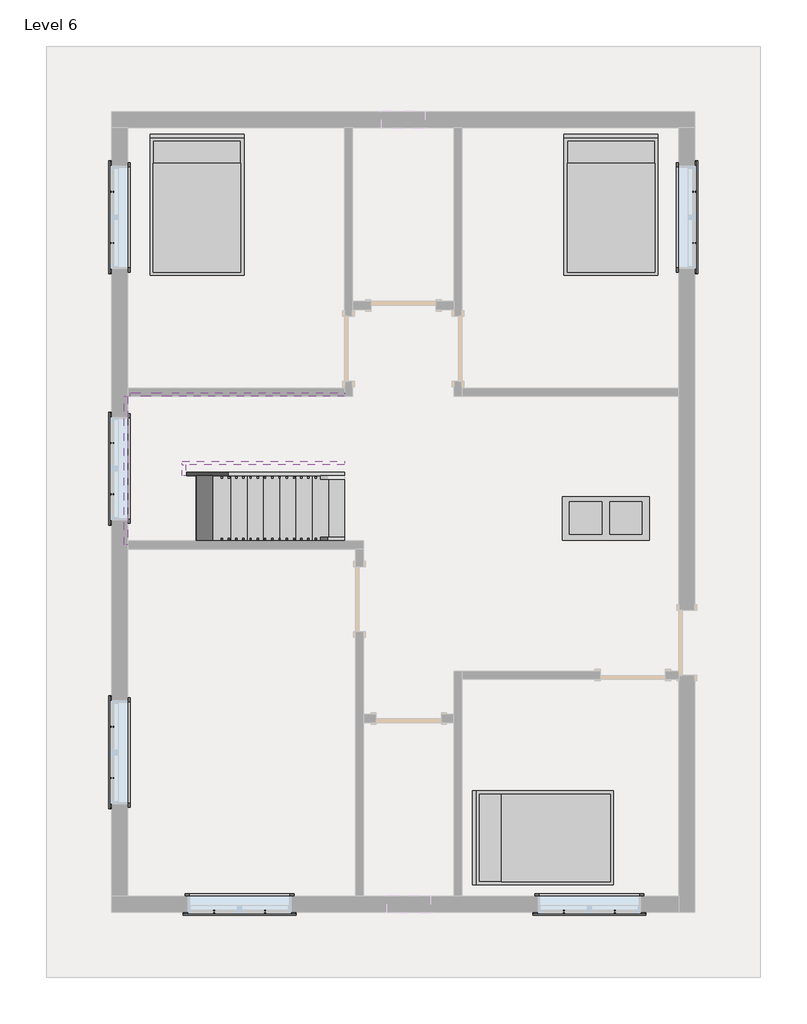
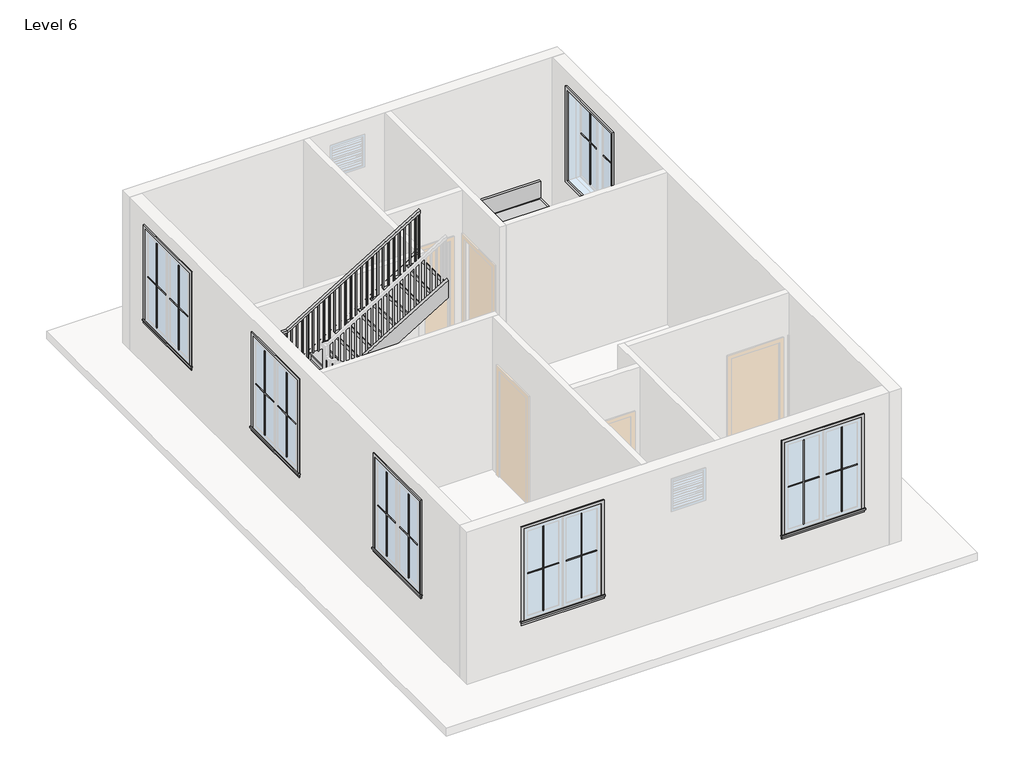
# One storey, part 2 of 2: 25 proxies, 6 members, 3 furniture elements, 1 railing, 1 stair flight.
"""IFC4 building model written with IfcOpenShell, lengths in millimetres."""

from ifc_helpers import new_model, si_unit, frame, origin, place, context, project, spatial, polyline, outline, extrude, faceted_brep, transform, mapped, element, save
from components import muntin_pattern_2x2_muntin_pattern_2x2_bff912c5, muntin_pattern_2x2_muntin_pattern_2x2_c2194282, trim_window_exterior_flat_with_sill_e04b3088, trim_window_interior_flat_picture_frame_2a7685fe, coffee_table_with_brass_mullions_11320_coffee_table_with_5962bef7, bed_17739_bed_17739_15c61121, stair_flight_418e8841

model = new_model("IFC4")

# Units and contexts
model_context = context("Model", 3, world=origin())
ifc_project = project(units=[si_unit("LENGTHUNIT", "METRE", prefix="MILLI")], contexts=[model_context])

# Site, building, storey
site = spatial("IfcSite", under=ifc_project)
building = spatial("IfcBuilding", under=site)
storey = spatial("IfcBuildingStorey", under=building, Name="Level 6", Elevation=12801.6)

# Proxies
placement = place(None, origin())
muntin_pattern_2x2_muntin_pattern_2x2_shape = muntin_pattern_2x2_muntin_pattern_2x2_bff912c5(model_context)
element("IfcBuildingElementProxy", 1, Name="Muntin Pattern_2x2 : Muntin Pattern_2x2", ObjectType="Muntin Pattern_2x2 : Muntin Pattern_2x2", at=placement, inside=storey, context=model_context, shape_type="MappedRepresentation", body=[
    mapped(muntin_pattern_2x2_muntin_pattern_2x2_shape, transform((-3196.8535855, -5792.3946383, 13785.85), x_axis=(-1.0, 0.0, 0.0), y_axis=(0.0, -1.0, 0.0), z_axis=(0.0, 0.0, 1.0))),
])
element("IfcBuildingElementProxy", 2, Name="Muntin Pattern_2x2 : Muntin Pattern_2x2", ObjectType="Muntin Pattern_2x2 : Muntin Pattern_2x2", at=placement, inside=storey, context=model_context, shape_type="MappedRepresentation", body=[
    mapped(muntin_pattern_2x2_muntin_pattern_2x2_shape, transform((-5347.9160855, -3914.3821383, 13785.85), x_axis=(0.0, 1.0, 0.0), y_axis=(-1.0, 0.0, 0.0), z_axis=(0.0, 0.0, 1.0))),
])
element("IfcBuildingElementProxy", 3, Name="Muntin Pattern_2x2 : Muntin Pattern_2x2", ObjectType="Muntin Pattern_2x2 : Muntin Pattern_2x2", at=placement, inside=storey, context=model_context, shape_type="MappedRepresentation", body=[
    mapped(muntin_pattern_2x2_muntin_pattern_2x2_shape, transform((1721.2214145, -5792.3946383, 13785.85), x_axis=(-1.0, 0.0, 0.0), y_axis=(0.0, -1.0, 0.0), z_axis=(0.0, 0.0, 1.0))),
])
element("IfcBuildingElementProxy", 4, Name="Muntin Pattern_2x2 : Muntin Pattern_2x2", ObjectType="Muntin Pattern_2x2 : Muntin Pattern_2x2", at=placement, inside=storey, context=model_context, shape_type="MappedRepresentation", body=[
    mapped(muntin_pattern_2x2_muntin_pattern_2x2_shape, transform((2837.2339145, 4324.7428617, 13785.85), x_axis=(0.0, -1.0, 0.0), y_axis=(1.0, 0.0, 0.0), z_axis=(0.0, 0.0, 1.0))),
])
element("IfcBuildingElementProxy", 5, Name="Muntin Pattern_2x2 : Muntin Pattern_2x2", ObjectType="Muntin Pattern_2x2 : Muntin Pattern_2x2", at=placement, inside=storey, context=model_context, shape_type="MappedRepresentation", body=[
    mapped(muntin_pattern_2x2_muntin_pattern_2x2_shape, transform((-5347.9160855, 3604.0178617, 13785.85), x_axis=(0.0, 1.0, 0.0), y_axis=(-1.0, 0.0, 0.0), z_axis=(0.0, 0.0, 1.0))),
])
element("IfcBuildingElementProxy", 6, Name="Muntin Pattern_2x2 : Muntin Pattern_2x2", ObjectType="Muntin Pattern_2x2 : Muntin Pattern_2x2", at=placement, inside=storey, context=model_context, shape_type="MappedRepresentation", body=[
    mapped(muntin_pattern_2x2_muntin_pattern_2x2_shape, transform((-5347.9160855, 73.4178617, 13785.85), x_axis=(0.0, 1.0, 0.0), y_axis=(-1.0, 0.0, 0.0), z_axis=(0.0, 0.0, 1.0))),
])
muntin_pattern_2x2_muntin_pattern_2x2_2_shape = muntin_pattern_2x2_muntin_pattern_2x2_c2194282(model_context)
element("IfcBuildingElementProxy", 7, Name="Muntin Pattern_2x2 : Muntin Pattern_2x2", ObjectType="Muntin Pattern_2x2 : Muntin Pattern_2x2", at=placement, inside=storey, context=model_context, shape_type="MappedRepresentation", body=[
    mapped(muntin_pattern_2x2_muntin_pattern_2x2_2_shape, transform((-3917.5785855, -5792.3946383, 13785.85), x_axis=(1.0, 0.0, 0.0), y_axis=(0.0, 1.0, 0.0), z_axis=(0.0, 0.0, 1.0))),
])
element("IfcBuildingElementProxy", 8, Name="Muntin Pattern_2x2 : Muntin Pattern_2x2", ObjectType="Muntin Pattern_2x2 : Muntin Pattern_2x2", at=placement, inside=storey, context=model_context, shape_type="MappedRepresentation", body=[
    mapped(muntin_pattern_2x2_muntin_pattern_2x2_2_shape, transform((-5347.9160855, -3193.6571383, 13785.85), x_axis=(0.0, -1.0, 0.0), y_axis=(1.0, 0.0, 0.0), z_axis=(0.0, 0.0, 1.0))),
])
element("IfcBuildingElementProxy", 9, Name="Muntin Pattern_2x2 : Muntin Pattern_2x2", ObjectType="Muntin Pattern_2x2 : Muntin Pattern_2x2", at=placement, inside=storey, context=model_context, shape_type="MappedRepresentation", body=[
    mapped(muntin_pattern_2x2_muntin_pattern_2x2_2_shape, transform((1000.4964145, -5792.3946383, 13785.85), x_axis=(1.0, 0.0, 0.0), y_axis=(0.0, 1.0, 0.0), z_axis=(0.0, 0.0, 1.0))),
])
element("IfcBuildingElementProxy", 10, Name="Muntin Pattern_2x2 : Muntin Pattern_2x2", ObjectType="Muntin Pattern_2x2 : Muntin Pattern_2x2", at=placement, inside=storey, context=model_context, shape_type="MappedRepresentation", body=[
    mapped(muntin_pattern_2x2_muntin_pattern_2x2_2_shape, transform((2837.2339145, 3604.0178617, 13785.85), x_axis=(0.0, 1.0, 0.0), y_axis=(-1.0, 0.0, 0.0), z_axis=(0.0, 0.0, 1.0))),
])
element("IfcBuildingElementProxy", 11, Name="Muntin Pattern_2x2 : Muntin Pattern_2x2", ObjectType="Muntin Pattern_2x2 : Muntin Pattern_2x2", at=placement, inside=storey, context=model_context, shape_type="MappedRepresentation", body=[
    mapped(muntin_pattern_2x2_muntin_pattern_2x2_2_shape, transform((-5347.9160855, 4324.7428617, 13785.85), x_axis=(0.0, -1.0, 0.0), y_axis=(1.0, 0.0, 0.0), z_axis=(0.0, 0.0, 1.0))),
])
element("IfcBuildingElementProxy", 12, Name="Muntin Pattern_2x2 : Muntin Pattern_2x2", ObjectType="Muntin Pattern_2x2 : Muntin Pattern_2x2", at=placement, inside=storey, context=model_context, shape_type="MappedRepresentation", body=[
    mapped(muntin_pattern_2x2_muntin_pattern_2x2_2_shape, transform((-5347.9160855, 794.1428617, 13785.85), x_axis=(0.0, -1.0, 0.0), y_axis=(1.0, 0.0, 0.0), z_axis=(0.0, 0.0, 1.0))),
])
trim_window_exterior_flat_with_sill_shape = trim_window_exterior_flat_with_sill_e04b3088(model_context)
element("IfcBuildingElementProxy", 13, Name="Trim-Window-Exterior-Flat : with Sill", ObjectType="Trim-Window-Exterior-Flat : with Sill", at=placement, inside=storey, context=model_context, shape_type="MappedRepresentation", body=[
    mapped(trim_window_exterior_flat_with_sill_shape, transform((-3557.2160855, -5801.9196383, 15544.8), x_axis=(1.0, 0.0, 0.0), y_axis=(0.0, 0.0, 1.0), z_axis=(0.0, -1.0, 0.0))),
])
element("IfcBuildingElementProxy", 14, Name="Trim-Window-Exterior-Flat : with Sill", ObjectType="Trim-Window-Exterior-Flat : with Sill", at=placement, inside=storey, context=model_context, shape_type="MappedRepresentation", body=[
    mapped(trim_window_exterior_flat_with_sill_shape, transform((-5357.4410855, -3554.0196383, 15544.8), x_axis=(0.0, -1.0, 0.0), y_axis=(0.0, 0.0, 1.0), z_axis=(-1.0, 0.0, 0.0))),
])
element("IfcBuildingElementProxy", 15, Name="Trim-Window-Exterior-Flat : with Sill", ObjectType="Trim-Window-Exterior-Flat : with Sill", at=placement, inside=storey, context=model_context, shape_type="MappedRepresentation", body=[
    mapped(trim_window_exterior_flat_with_sill_shape, transform((1360.8589145, -5801.9196383, 15544.8), x_axis=(1.0, 0.0, 0.0), y_axis=(0.0, 0.0, 1.0), z_axis=(0.0, -1.0, 0.0))),
])
element("IfcBuildingElementProxy", 16, Name="Trim-Window-Exterior-Flat : with Sill", ObjectType="Trim-Window-Exterior-Flat : with Sill", at=placement, inside=storey, context=model_context, shape_type="MappedRepresentation", body=[
    mapped(trim_window_exterior_flat_with_sill_shape, transform((2846.7589145, 3964.3803617, 15544.8), x_axis=(0.0, 1.0, 0.0), y_axis=(0.0, 0.0, 1.0), z_axis=(1.0, 0.0, 0.0))),
])
element("IfcBuildingElementProxy", 17, Name="Trim-Window-Exterior-Flat : with Sill", ObjectType="Trim-Window-Exterior-Flat : with Sill", at=placement, inside=storey, context=model_context, shape_type="MappedRepresentation", body=[
    mapped(trim_window_exterior_flat_with_sill_shape, transform((-5357.4410855, 3964.3803617, 15544.8), x_axis=(0.0, -1.0, 0.0), y_axis=(0.0, 0.0, 1.0), z_axis=(-1.0, 0.0, 0.0))),
])
element("IfcBuildingElementProxy", 18, Name="Trim-Window-Exterior-Flat : with Sill", ObjectType="Trim-Window-Exterior-Flat : with Sill", at=placement, inside=storey, context=model_context, shape_type="MappedRepresentation", body=[
    mapped(trim_window_exterior_flat_with_sill_shape, transform((-5357.4410855, 433.7803617, 15544.8), x_axis=(0.0, -1.0, 0.0), y_axis=(0.0, 0.0, 1.0), z_axis=(-1.0, 0.0, 0.0))),
])
trim_window_interior_flat_picture_frame_shape = trim_window_interior_flat_picture_frame_2a7685fe(model_context)
element("IfcBuildingElementProxy", 19, Name="Trim-Window-Interior-Flat : Picture Frame", ObjectType="Trim-Window-Interior-Flat : Picture Frame", at=placement, inside=storey, context=model_context, shape_type="MappedRepresentation", body=[
    mapped(trim_window_interior_flat_picture_frame_shape, transform((-3557.2160855, -5573.3196383, 15544.8), x_axis=(-1.0, 0.0, 0.0), y_axis=(0.0, 0.0, 1.0), z_axis=(0.0, 1.0, 0.0))),
])
element("IfcBuildingElementProxy", 20, Name="Trim-Window-Interior-Flat : Picture Frame", ObjectType="Trim-Window-Interior-Flat : Picture Frame", at=placement, inside=storey, context=model_context, shape_type="MappedRepresentation", body=[
    mapped(trim_window_interior_flat_picture_frame_shape, transform((-5128.8410855, -3554.0196383, 15544.8), x_axis=(0.0, 1.0, 0.0), y_axis=(0.0, 0.0, 1.0), z_axis=(1.0, 0.0, 0.0))),
])
element("IfcBuildingElementProxy", 21, Name="Trim-Window-Interior-Flat : Picture Frame", ObjectType="Trim-Window-Interior-Flat : Picture Frame", at=placement, inside=storey, context=model_context, shape_type="MappedRepresentation", body=[
    mapped(trim_window_interior_flat_picture_frame_shape, transform((1360.8589145, -5573.3196383, 15544.8), x_axis=(-1.0, 0.0, 0.0), y_axis=(0.0, 0.0, 1.0), z_axis=(0.0, 1.0, 0.0))),
])
element("IfcBuildingElementProxy", 22, Name="Trim-Window-Interior-Flat : Picture Frame", ObjectType="Trim-Window-Interior-Flat : Picture Frame", at=placement, inside=storey, context=model_context, shape_type="MappedRepresentation", body=[
    mapped(trim_window_interior_flat_picture_frame_shape, transform((2618.1589145, 3964.3803617, 15544.8), x_axis=(0.0, -1.0, 0.0), y_axis=(0.0, 0.0, 1.0), z_axis=(-1.0, 0.0, 0.0))),
])
element("IfcBuildingElementProxy", 23, Name="Trim-Window-Interior-Flat : Picture Frame", ObjectType="Trim-Window-Interior-Flat : Picture Frame", at=placement, inside=storey, context=model_context, shape_type="MappedRepresentation", body=[
    mapped(trim_window_interior_flat_picture_frame_shape, transform((-5128.8410855, 3964.3803617, 15544.8), x_axis=(0.0, 1.0, 0.0), y_axis=(0.0, 0.0, 1.0), z_axis=(1.0, 0.0, 0.0))),
])
element("IfcBuildingElementProxy", 24, Name="Trim-Window-Interior-Flat : Picture Frame", ObjectType="Trim-Window-Interior-Flat : Picture Frame", at=placement, inside=storey, context=model_context, shape_type="MappedRepresentation", body=[
    mapped(trim_window_interior_flat_picture_frame_shape, transform((-5128.8410855, 433.7803617, 15544.8), x_axis=(0.0, 1.0, 0.0), y_axis=(0.0, 0.0, 1.0), z_axis=(1.0, 0.0, 0.0))),
])
coffee_table_with_brass_mullions_11320_coffee_table_with_shape = coffee_table_with_brass_mullions_11320_coffee_table_with_5962bef7(model_context)
element("IfcBuildingElementProxy", 25, Name="coffee_table_with_brass_mullions_11320 : coffee_table_with_brass_mullions_11320", ObjectType="coffee_table_with_brass_mullions_11320 : coffee_table_with_brass_mullions_11320", at=placement, inside=storey, context=model_context, shape_type="MappedRepresentation", body=[
    mapped(coffee_table_with_brass_mullions_11320_coffee_table_with_shape, transform((2229.2258874, -696.5196383, 12801.6), x_axis=(1.0, 0.0, 0.0), y_axis=(0.0, 1.0, 0.0), z_axis=(0.0, 0.0, 1.0))),
])

# Furniture
bed_17739_bed_17739_shape = bed_17739_bed_17739_15c61121(model_context)
element("IfcFurniture", 26, ObjectType="Bed_17739 : Bed_17739", at=placement, inside=storey, context=model_context, shape_type="MappedRepresentation", body=[
    mapped(bed_17739_bed_17739_shape, transform((1665.6589145, 4116.7803617, 12801.6), x_axis=(1.0, 0.0, 0.0), y_axis=(0.0, 1.0, 0.0), z_axis=(0.0, 0.0, 1.0))),
])
element("IfcFurniture", 27, ObjectType="Bed_17739 : Bed_17739", at=placement, inside=storey, context=model_context, shape_type="MappedRepresentation", body=[
    mapped(bed_17739_bed_17739_shape, transform((-4157.2910855, 4116.7803617, 12801.6), x_axis=(1.0, 0.0, 0.0), y_axis=(0.0, 1.0, 0.0), z_axis=(0.0, 0.0, 1.0))),
])
element("IfcFurniture", 28, ObjectType="Bed_17739 : Bed_17739", at=placement, inside=storey, context=model_context, shape_type="MappedRepresentation", body=[
    mapped(bed_17739_bed_17739_shape, transform((732.2089145, -4754.5725945, 12801.6), x_axis=(0.0, 1.0, 0.0), y_axis=(-1.0, 0.0, 0.0), z_axis=(0.0, 0.0, 1.0))),
])

# Members
element("IfcMember", 29, ObjectType="Stringer - 2\" Width", at=placement, inside=storey, context=model_context, shape_type="SweptSolid", body=[
    extrude(outline(polyline([(12801.6, -2080.8410855), (13013.714512, -2080.8410855), (14401.8, -4371.1821407), (14401.8, -4959.2565972), (12801.6, -2318.9265972), (12801.6, -2080.8410855)])), frame((0.0, -633.0196383, 0.0), z_axis=(0.0, 1.0, 0.0), x_axis=(0.0, 0.0, 1.0)), (0.0, 0.0, 1.0), 50.8),
])
element("IfcMember", 30, ObjectType="Stringer - 2\" Width", at=placement, inside=storey, context=model_context, shape_type="SweptSolid", body=[
    extrude(outline(polyline([(-5128.8410855, -633.0196383), (-5179.6410855, -633.0196383), (-5179.6410855, 1449.7803617), (-5128.8410855, 1449.7803617), (-5128.8410855, -633.0196383)])), frame((0.0, 0.0, 14097.0), z_axis=(0.0, 0.0, 1.0), x_axis=(1.0, 0.0, 0.0)), (0.0, 0.0, 1.0), 304.8),
])
element("IfcMember", 31, ObjectType="Stringer - 2\" Width", at=placement, inside=storey, context=model_context, shape_type="SweptSolid", body=[
    extrude(outline(polyline([(14097.0, -4505.9455737), (15566.7602959, -2080.8410855), (15923.1690574, -2080.8410855), (14097.0, -5094.0200302), (14097.0, -4505.9455737)])), frame((0.0, 1449.7803617, 0.0), z_axis=(0.0, 1.0, 0.0), x_axis=(0.0, 0.0, 1.0)), (0.0, 0.0, 1.0), 50.8),
])
element("IfcMember", 32, ObjectType="Stringer - 2\" Width", at=placement, inside=storey, context=model_context, shape_type="SweptSolid", body=[
    extrude(outline(polyline([(12801.6, -2080.8410855), (13013.714512, -2080.8410855), (14368.3811786, -4316.0410855), (14011.9724171, -4316.0410855), (12801.6, -2318.9265972), (12801.6, -2080.8410855)])), frame((0.0, 332.1803617, 0.0), z_axis=(0.0, 1.0, 0.0), x_axis=(0.0, 0.0, 1.0)), (0.0, 0.0, 1.0), 50.8),
])
element("IfcMember", 33, ObjectType="Stringer - 2\" Width", at=placement, inside=storey, context=model_context, shape_type="SweptSolid", body=[
    extrude(outline(polyline([(-4316.0410855, 332.1803617), (-4366.8410855, 332.1803617), (-4366.8410855, 484.5803617), (-4316.0410855, 484.5803617), (-4316.0410855, 332.1803617)])), frame((0.0, 0.0, 14097.0), z_axis=(0.0, 0.0, 1.0), x_axis=(1.0, 0.0, 0.0)), (0.0, 0.0, 1.0), 304.8),
])
element("IfcMember", 34, ObjectType="Stringer - 2\" Width", at=placement, inside=storey, context=model_context, shape_type="SweptSolid", body=[
    extrude(outline(polyline([(14537.714512, -4366.8410855), (14181.3057504, -4366.8410855), (15566.7602959, -2080.8410855), (15923.1690574, -2080.8410855), (14537.714512, -4366.8410855)])), frame((0.0, 484.5803617, 0.0), z_axis=(0.0, 1.0, 0.0), x_axis=(0.0, 0.0, 1.0)), (0.0, 0.0, 1.0), 50.8),
])

# Railing
element("IfcRailing", 35, ObjectType="Handrail - Rectangular", at=placement, inside=storey, context=model_context, shape_type="SolidModel", body=[
    faceted_brep([(-2080.8410855, -582.2196383, 13854.5454545), (-2080.8410855, -582.2196383, 13795.1439943), (-2080.8410855, -531.4196383, 13795.1439943), (-2080.8410855, -531.4196383, 13854.5454545), (-4366.8410855, -582.2196383, 15240.0), (-4381.0334949, -582.2196383, 15189.2), (-4381.0334949, -531.4196383, 15189.2), (-4366.8410855, -531.4196383, 15240.0), (-5128.8410855, -582.2196383, 15240.0), (-5128.8410855, -582.2196383, 15189.2), (-5078.0410855, -531.4196383, 15189.2), (-5078.0410855, -531.4196383, 15240.0), (-5128.8410855, 1449.7803617, 15240.0), (-5128.8410855, 1449.7803617, 15189.2), (-5078.0410855, 1398.9803617, 15189.2), (-5078.0410855, 1398.9803617, 15240.0), (-4595.4410855, 1449.7803617, 15240.0), (-4581.2486761, 1449.7803617, 15189.2), (-4581.2486761, 1398.9803617, 15189.2), (-4595.4410855, 1398.9803617, 15240.0), (-2080.8410855, 1449.7803617, 16764.0), (-2080.8410855, 1398.9803617, 16764.0), (-2080.8410855, 1398.9803617, 16704.5985397), (-2080.8410855, 1449.7803617, 16704.5985397)], [[[0, 1, 2, 3]], [[1, 0, 4, 5]], [[2, 1, 5, 6]], [[3, 2, 6, 7]], [[0, 3, 7, 4]], [[5, 4, 8, 9]], [[6, 5, 9, 10]], [[7, 6, 10, 11]], [[4, 7, 11, 8]], [[9, 8, 12, 13]], [[10, 9, 13, 14]], [[11, 10, 14, 15]], [[8, 11, 15, 12]], [[13, 12, 16, 17]], [[14, 13, 17, 18]], [[15, 14, 18, 19]], [[12, 15, 19, 16]], [[20, 21, 22, 23]], [[17, 16, 20, 23]], [[18, 17, 23, 22]], [[19, 18, 22, 21]], [[16, 19, 21, 20]]]),
    extrude(outline(polyline([(16652.6439943, -2166.5660855), (15711.0545455, -2166.5660855), (15711.0545455, -2147.5160855), (16664.1894488, -2147.5160855), (16652.6439943, -2166.5660855)])), frame((0.0, 1414.8553617, 0.0), z_axis=(0.0, 1.0, 0.0), x_axis=(0.0, 0.0, 1.0)), (0.0, 0.0, 1.0), 19.05),
    extrude(outline(polyline([(16591.0682367, -2268.1660855), (15711.0545455, -2268.1660855), (15711.0545455, -2249.1160855), (16602.6136913, -2249.1160855), (16591.0682367, -2268.1660855)])), frame((0.0, 1414.8553617, 0.0), z_axis=(0.0, 1.0, 0.0), x_axis=(0.0, 0.0, 1.0)), (0.0, 0.0, 1.0), 19.05),
    extrude(outline(polyline([(16529.4924791, -2369.7660855), (15572.5090909, -2369.7660855), (15572.5090909, -2350.7160855), (16541.0379337, -2350.7160855), (16529.4924791, -2369.7660855)])), frame((0.0, 1414.8553617, 0.0), z_axis=(0.0, 1.0, 0.0), x_axis=(0.0, 0.0, 1.0)), (0.0, 0.0, 1.0), 19.05),
    extrude(outline(polyline([(16467.9167216, -2471.3660855), (15572.5090909, -2471.3660855), (15572.5090909, -2452.3160855), (16479.4621761, -2452.3160855), (16467.9167216, -2471.3660855)])), frame((0.0, 1414.8553617, 0.0), z_axis=(0.0, 1.0, 0.0), x_axis=(0.0, 0.0, 1.0)), (0.0, 0.0, 1.0), 19.05),
    extrude(outline(polyline([(16406.340964, -2572.9660855), (15433.9636364, -2572.9660855), (15433.9636364, -2553.9160855), (16417.8864185, -2553.9160855), (16406.340964, -2572.9660855)])), frame((0.0, 1414.8553617, 0.0), z_axis=(0.0, 1.0, 0.0), x_axis=(0.0, 0.0, 1.0)), (0.0, 0.0, 1.0), 19.05),
    extrude(outline(polyline([(16344.7652064, -2674.5660855), (15433.9636364, -2674.5660855), (15433.9636364, -2655.5160855), (16356.310661, -2655.5160855), (16344.7652064, -2674.5660855)])), frame((0.0, 1414.8553617, 0.0), z_axis=(0.0, 1.0, 0.0), x_axis=(0.0, 0.0, 1.0)), (0.0, 0.0, 1.0), 19.05),
    extrude(outline(polyline([(16283.1894488, -2776.1660855), (15433.9636364, -2776.1660855), (15433.9636364, -2757.1160855), (16294.7349034, -2757.1160855), (16283.1894488, -2776.1660855)])), frame((0.0, 1414.8553617, 0.0), z_axis=(0.0, 1.0, 0.0), x_axis=(0.0, 0.0, 1.0)), (0.0, 0.0, 1.0), 19.05),
    extrude(outline(polyline([(16221.6136913, -2877.7660855), (15295.4181818, -2877.7660855), (15295.4181818, -2858.7160855), (16233.1591458, -2858.7160855), (16221.6136913, -2877.7660855)])), frame((0.0, 1414.8553617, 0.0), z_axis=(0.0, 1.0, 0.0), x_axis=(0.0, 0.0, 1.0)), (0.0, 0.0, 1.0), 19.05),
    extrude(outline(polyline([(16160.0379337, -2979.3660855), (15295.4181818, -2979.3660855), (15295.4181818, -2960.3160855), (16171.5833882, -2960.3160855), (16160.0379337, -2979.3660855)])), frame((0.0, 1414.8553617, 0.0), z_axis=(0.0, 1.0, 0.0), x_axis=(0.0, 0.0, 1.0)), (0.0, 0.0, 1.0), 19.05),
    extrude(outline(polyline([(16098.4621761, -3080.9660855), (15156.8727273, -3080.9660855), (15156.8727273, -3061.9160855), (16110.0076307, -3061.9160855), (16098.4621761, -3080.9660855)])), frame((0.0, 1414.8553617, 0.0), z_axis=(0.0, 1.0, 0.0), x_axis=(0.0, 0.0, 1.0)), (0.0, 0.0, 1.0), 19.05),
    extrude(outline(polyline([(16036.8864185, -3182.5660855), (15156.8727273, -3182.5660855), (15156.8727273, -3163.5160855), (16048.4318731, -3163.5160855), (16036.8864185, -3182.5660855)])), frame((0.0, 1414.8553617, 0.0), z_axis=(0.0, 1.0, 0.0), x_axis=(0.0, 0.0, 1.0)), (0.0, 0.0, 1.0), 19.05),
    extrude(outline(polyline([(15975.310661, -3284.1660855), (15018.3272727, -3284.1660855), (15018.3272727, -3265.1160855), (15986.8561155, -3265.1160855), (15975.310661, -3284.1660855)])), frame((0.0, 1414.8553617, 0.0), z_axis=(0.0, 1.0, 0.0), x_axis=(0.0, 0.0, 1.0)), (0.0, 0.0, 1.0), 19.05),
    extrude(outline(polyline([(15913.7349034, -3385.7660855), (15018.3272727, -3385.7660855), (15018.3272727, -3366.7160855), (15925.2803579, -3366.7160855), (15913.7349034, -3385.7660855)])), frame((0.0, 1414.8553617, 0.0), z_axis=(0.0, 1.0, 0.0), x_axis=(0.0, 0.0, 1.0)), (0.0, 0.0, 1.0), 19.05),
    extrude(outline(polyline([(15852.1591458, -3487.3660855), (14879.7818182, -3487.3660855), (14879.7818182, -3468.3160855), (15863.7046004, -3468.3160855), (15852.1591458, -3487.3660855)])), frame((0.0, 1414.8553617, 0.0), z_axis=(0.0, 1.0, 0.0), x_axis=(0.0, 0.0, 1.0)), (0.0, 0.0, 1.0), 19.05),
    extrude(outline(polyline([(15790.5833882, -3588.9660855), (14879.7818182, -3588.9660855), (14879.7818182, -3569.9160855), (15802.1288428, -3569.9160855), (15790.5833882, -3588.9660855)])), frame((0.0, 1414.8553617, 0.0), z_axis=(0.0, 1.0, 0.0), x_axis=(0.0, 0.0, 1.0)), (0.0, 0.0, 1.0), 19.05),
    extrude(outline(polyline([(15729.0076307, -3690.5660855), (14879.7818182, -3690.5660855), (14879.7818182, -3671.5160855), (15740.5530852, -3671.5160855), (15729.0076307, -3690.5660855)])), frame((0.0, 1414.8553617, 0.0), z_axis=(0.0, 1.0, 0.0), x_axis=(0.0, 0.0, 1.0)), (0.0, 0.0, 1.0), 19.05),
    extrude(outline(polyline([(15667.4318731, -3792.1660855), (14741.2363636, -3792.1660855), (14741.2363636, -3773.1160855), (15678.9773276, -3773.1160855), (15667.4318731, -3792.1660855)])), frame((0.0, 1414.8553617, 0.0), z_axis=(0.0, 1.0, 0.0), x_axis=(0.0, 0.0, 1.0)), (0.0, 0.0, 1.0), 19.05),
    extrude(outline(polyline([(15605.8561155, -3893.7660855), (14741.2363636, -3893.7660855), (14741.2363636, -3874.7160855), (15617.40157, -3874.7160855), (15605.8561155, -3893.7660855)])), frame((0.0, 1414.8553617, 0.0), z_axis=(0.0, 1.0, 0.0), x_axis=(0.0, 0.0, 1.0)), (0.0, 0.0, 1.0), 19.05),
    extrude(outline(polyline([(15544.2803579, -3995.3660855), (14602.6909091, -3995.3660855), (14602.6909091, -3976.3160855), (15555.8258125, -3976.3160855), (15544.2803579, -3995.3660855)])), frame((0.0, 1414.8553617, 0.0), z_axis=(0.0, 1.0, 0.0), x_axis=(0.0, 0.0, 1.0)), (0.0, 0.0, 1.0), 19.05),
    extrude(outline(polyline([(15482.7046004, -4096.9660855), (14602.6909091, -4096.9660855), (14602.6909091, -4077.9160855), (15494.2500549, -4077.9160855), (15482.7046004, -4096.9660855)])), frame((0.0, 1414.8553617, 0.0), z_axis=(0.0, 1.0, 0.0), x_axis=(0.0, 0.0, 1.0)), (0.0, 0.0, 1.0), 19.05),
    extrude(outline(polyline([(15421.1288428, -4198.5660855), (14464.1454545, -4198.5660855), (14464.1454545, -4179.5160855), (15432.6742973, -4179.5160855), (15421.1288428, -4198.5660855)])), frame((0.0, 1414.8553617, 0.0), z_axis=(0.0, 1.0, 0.0), x_axis=(0.0, 0.0, 1.0)), (0.0, 0.0, 1.0), 19.05),
    extrude(outline(polyline([(15359.5530852, -4300.1660855), (14464.1454545, -4300.1660855), (14464.1454545, -4281.1160855), (15371.0985397, -4281.1160855), (15359.5530852, -4300.1660855)])), frame((0.0, 1414.8553617, 0.0), z_axis=(0.0, 1.0, 0.0), x_axis=(0.0, 0.0, 1.0)), (0.0, 0.0, 1.0), 19.05),
    extrude(outline(polyline([(15297.9773276, -4401.7660855), (14325.6, -4401.7660855), (14325.6, -4382.7160855), (15309.5227822, -4382.7160855), (15297.9773276, -4401.7660855)])), frame((0.0, 1414.8553617, 0.0), z_axis=(0.0, 1.0, 0.0), x_axis=(0.0, 0.0, 1.0)), (0.0, 0.0, 1.0), 19.05),
    extrude(outline(polyline([(15236.40157, -4503.3660855), (14325.6, -4503.3660855), (14325.6, -4484.3160855), (15247.9470246, -4484.3160855), (15236.40157, -4503.3660855)])), frame((0.0, 1414.8553617, 0.0), z_axis=(0.0, 1.0, 0.0), x_axis=(0.0, 0.0, 1.0)), (0.0, 0.0, 1.0), 19.05),
    extrude(outline(polyline([(-4604.9660855, 1433.9053617), (-4585.9160855, 1433.9053617), (-4585.9160855, 1414.8553617), (-4604.9660855, 1414.8553617), (-4604.9660855, 1433.9053617)])), frame((0.0, 0.0, 14325.6), z_axis=(0.0, 0.0, 1.0), x_axis=(1.0, 0.0, 0.0)), (0.0, 0.0, 1.0), 863.6),
    extrude(outline(polyline([(-4706.5660855, 1433.9053617), (-4687.5160855, 1433.9053617), (-4687.5160855, 1414.8553617), (-4706.5660855, 1414.8553617), (-4706.5660855, 1433.9053617)])), frame((0.0, 0.0, 14325.6), z_axis=(0.0, 0.0, 1.0), x_axis=(1.0, 0.0, 0.0)), (0.0, 0.0, 1.0), 863.6),
    extrude(outline(polyline([(-4808.1660855, 1433.9053617), (-4789.1160855, 1433.9053617), (-4789.1160855, 1414.8553617), (-4808.1660855, 1414.8553617), (-4808.1660855, 1433.9053617)])), frame((0.0, 0.0, 14325.6), z_axis=(0.0, 0.0, 1.0), x_axis=(1.0, 0.0, 0.0)), (0.0, 0.0, 1.0), 863.6),
    extrude(outline(polyline([(-4909.7660855, 1433.9053617), (-4890.7160855, 1433.9053617), (-4890.7160855, 1414.8553617), (-4909.7660855, 1414.8553617), (-4909.7660855, 1433.9053617)])), frame((0.0, 0.0, 14325.6), z_axis=(0.0, 0.0, 1.0), x_axis=(1.0, 0.0, 0.0)), (0.0, 0.0, 1.0), 863.6),
    extrude(outline(polyline([(-5011.3660855, 1433.9053617), (-4992.3160855, 1433.9053617), (-4992.3160855, 1414.8553617), (-5011.3660855, 1414.8553617), (-5011.3660855, 1433.9053617)])), frame((0.0, 0.0, 14325.6), z_axis=(0.0, 0.0, 1.0), x_axis=(1.0, 0.0, 0.0)), (0.0, 0.0, 1.0), 863.6),
    extrude(outline(polyline([(-5112.9660855, 1364.0553617), (-5112.9660855, 1383.1053617), (-5093.9160855, 1383.1053617), (-5093.9160855, 1364.0553617), (-5112.9660855, 1364.0553617)])), frame((0.0, 0.0, 14325.6), z_axis=(0.0, 0.0, 1.0), x_axis=(1.0, 0.0, 0.0)), (0.0, 0.0, 1.0), 863.6),
    extrude(outline(polyline([(-5112.9660855, 1262.4553617), (-5112.9660855, 1281.5053617), (-5093.9160855, 1281.5053617), (-5093.9160855, 1262.4553617), (-5112.9660855, 1262.4553617)])), frame((0.0, 0.0, 14325.6), z_axis=(0.0, 0.0, 1.0), x_axis=(1.0, 0.0, 0.0)), (0.0, 0.0, 1.0), 863.6),
    extrude(outline(polyline([(-5112.9660855, 1160.8553617), (-5112.9660855, 1179.9053617), (-5093.9160855, 1179.9053617), (-5093.9160855, 1160.8553617), (-5112.9660855, 1160.8553617)])), frame((0.0, 0.0, 14325.6), z_axis=(0.0, 0.0, 1.0), x_axis=(1.0, 0.0, 0.0)), (0.0, 0.0, 1.0), 863.6),
    extrude(outline(polyline([(-5112.9660855, 1059.2553617), (-5112.9660855, 1078.3053617), (-5093.9160855, 1078.3053617), (-5093.9160855, 1059.2553617), (-5112.9660855, 1059.2553617)])), frame((0.0, 0.0, 14325.6), z_axis=(0.0, 0.0, 1.0), x_axis=(1.0, 0.0, 0.0)), (0.0, 0.0, 1.0), 863.6),
    extrude(outline(polyline([(-5112.9660855, 957.6553617), (-5112.9660855, 976.7053617), (-5093.9160855, 976.7053617), (-5093.9160855, 957.6553617), (-5112.9660855, 957.6553617)])), frame((0.0, 0.0, 14325.6), z_axis=(0.0, 0.0, 1.0), x_axis=(1.0, 0.0, 0.0)), (0.0, 0.0, 1.0), 863.6),
    extrude(outline(polyline([(-5112.9660855, 856.0553617), (-5112.9660855, 875.1053617), (-5093.9160855, 875.1053617), (-5093.9160855, 856.0553617), (-5112.9660855, 856.0553617)])), frame((0.0, 0.0, 14325.6), z_axis=(0.0, 0.0, 1.0), x_axis=(1.0, 0.0, 0.0)), (0.0, 0.0, 1.0), 863.6),
    extrude(outline(polyline([(-5112.9660855, 754.4553617), (-5112.9660855, 773.5053617), (-5093.9160855, 773.5053617), (-5093.9160855, 754.4553617), (-5112.9660855, 754.4553617)])), frame((0.0, 0.0, 14325.6), z_axis=(0.0, 0.0, 1.0), x_axis=(1.0, 0.0, 0.0)), (0.0, 0.0, 1.0), 863.6),
    extrude(outline(polyline([(-5112.9660855, 652.8553617), (-5112.9660855, 671.9053617), (-5093.9160855, 671.9053617), (-5093.9160855, 652.8553617), (-5112.9660855, 652.8553617)])), frame((0.0, 0.0, 14325.6), z_axis=(0.0, 0.0, 1.0), x_axis=(1.0, 0.0, 0.0)), (0.0, 0.0, 1.0), 863.6),
    extrude(outline(polyline([(-5112.9660855, 551.2553617), (-5112.9660855, 570.3053617), (-5093.9160855, 570.3053617), (-5093.9160855, 551.2553617), (-5112.9660855, 551.2553617)])), frame((0.0, 0.0, 14325.6), z_axis=(0.0, 0.0, 1.0), x_axis=(1.0, 0.0, 0.0)), (0.0, 0.0, 1.0), 863.6),
    extrude(outline(polyline([(-5112.9660855, 449.6553617), (-5112.9660855, 468.7053617), (-5093.9160855, 468.7053617), (-5093.9160855, 449.6553617), (-5112.9660855, 449.6553617)])), frame((0.0, 0.0, 14325.6), z_axis=(0.0, 0.0, 1.0), x_axis=(1.0, 0.0, 0.0)), (0.0, 0.0, 1.0), 863.6),
    extrude(outline(polyline([(-5112.9660855, 348.0553617), (-5112.9660855, 367.1053617), (-5093.9160855, 367.1053617), (-5093.9160855, 348.0553617), (-5112.9660855, 348.0553617)])), frame((0.0, 0.0, 14325.6), z_axis=(0.0, 0.0, 1.0), x_axis=(1.0, 0.0, 0.0)), (0.0, 0.0, 1.0), 863.6),
    extrude(outline(polyline([(-5112.9660855, 246.4553617), (-5112.9660855, 265.5053617), (-5093.9160855, 265.5053617), (-5093.9160855, 246.4553617), (-5112.9660855, 246.4553617)])), frame((0.0, 0.0, 14325.6), z_axis=(0.0, 0.0, 1.0), x_axis=(1.0, 0.0, 0.0)), (0.0, 0.0, 1.0), 863.6),
    extrude(outline(polyline([(-5112.9660855, 144.8553617), (-5112.9660855, 163.9053617), (-5093.9160855, 163.9053617), (-5093.9160855, 144.8553617), (-5112.9660855, 144.8553617)])), frame((0.0, 0.0, 14325.6), z_axis=(0.0, 0.0, 1.0), x_axis=(1.0, 0.0, 0.0)), (0.0, 0.0, 1.0), 863.6),
    extrude(outline(polyline([(-5112.9660855, 43.2553617), (-5112.9660855, 62.3053617), (-5093.9160855, 62.3053617), (-5093.9160855, 43.2553617), (-5112.9660855, 43.2553617)])), frame((0.0, 0.0, 14325.6), z_axis=(0.0, 0.0, 1.0), x_axis=(1.0, 0.0, 0.0)), (0.0, 0.0, 1.0), 863.6),
    extrude(outline(polyline([(-5112.9660855, -58.3446383), (-5112.9660855, -39.2946383), (-5093.9160855, -39.2946383), (-5093.9160855, -58.3446383), (-5112.9660855, -58.3446383)])), frame((0.0, 0.0, 14325.6), z_axis=(0.0, 0.0, 1.0), x_axis=(1.0, 0.0, 0.0)), (0.0, 0.0, 1.0), 863.6),
    extrude(outline(polyline([(-5112.9660855, -159.9446383), (-5112.9660855, -140.8946383), (-5093.9160855, -140.8946383), (-5093.9160855, -159.9446383), (-5112.9660855, -159.9446383)])), frame((0.0, 0.0, 14325.6), z_axis=(0.0, 0.0, 1.0), x_axis=(1.0, 0.0, 0.0)), (0.0, 0.0, 1.0), 863.6),
    extrude(outline(polyline([(-5112.9660855, -261.5446383), (-5112.9660855, -242.4946383), (-5093.9160855, -242.4946383), (-5093.9160855, -261.5446383), (-5112.9660855, -261.5446383)])), frame((0.0, 0.0, 14325.6), z_axis=(0.0, 0.0, 1.0), x_axis=(1.0, 0.0, 0.0)), (0.0, 0.0, 1.0), 863.6),
    extrude(outline(polyline([(-5112.9660855, -363.1446383), (-5112.9660855, -344.0946383), (-5093.9160855, -344.0946383), (-5093.9160855, -363.1446383), (-5112.9660855, -363.1446383)])), frame((0.0, 0.0, 14325.6), z_axis=(0.0, 0.0, 1.0), x_axis=(1.0, 0.0, 0.0)), (0.0, 0.0, 1.0), 863.6),
    extrude(outline(polyline([(-5112.9660855, -464.7446383), (-5112.9660855, -445.6946383), (-5093.9160855, -445.6946383), (-5093.9160855, -464.7446383), (-5112.9660855, -464.7446383)])), frame((0.0, 0.0, 14325.6), z_axis=(0.0, 0.0, 1.0), x_axis=(1.0, 0.0, 0.0)), (0.0, 0.0, 1.0), 863.6),
    extrude(outline(polyline([(-5017.7160855, -566.3446383), (-5036.7660855, -566.3446383), (-5036.7660855, -547.2946383), (-5017.7160855, -547.2946383), (-5017.7160855, -566.3446383)])), frame((0.0, 0.0, 14325.6), z_axis=(0.0, 0.0, 1.0), x_axis=(1.0, 0.0, 0.0)), (0.0, 0.0, 1.0), 863.6),
    extrude(outline(polyline([(-4916.1160855, -566.3446383), (-4935.1660855, -566.3446383), (-4935.1660855, -547.2946383), (-4916.1160855, -547.2946383), (-4916.1160855, -566.3446383)])), frame((0.0, 0.0, 14325.6), z_axis=(0.0, 0.0, 1.0), x_axis=(1.0, 0.0, 0.0)), (0.0, 0.0, 1.0), 863.6),
    extrude(outline(polyline([(-4814.5160855, -566.3446383), (-4833.5660855, -566.3446383), (-4833.5660855, -547.2946383), (-4814.5160855, -547.2946383), (-4814.5160855, -566.3446383)])), frame((0.0, 0.0, 14325.6), z_axis=(0.0, 0.0, 1.0), x_axis=(1.0, 0.0, 0.0)), (0.0, 0.0, 1.0), 863.6),
    extrude(outline(polyline([(-4712.9160855, -566.3446383), (-4731.9660855, -566.3446383), (-4731.9660855, -547.2946383), (-4712.9160855, -547.2946383), (-4712.9160855, -566.3446383)])), frame((0.0, 0.0, 14325.6), z_axis=(0.0, 0.0, 1.0), x_axis=(1.0, 0.0, 0.0)), (0.0, 0.0, 1.0), 863.6),
    extrude(outline(polyline([(-4611.3160855, -566.3446383), (-4630.3660855, -566.3446383), (-4630.3660855, -547.2946383), (-4611.3160855, -547.2946383), (-4611.3160855, -566.3446383)])), frame((0.0, 0.0, 14325.6), z_axis=(0.0, 0.0, 1.0), x_axis=(1.0, 0.0, 0.0)), (0.0, 0.0, 1.0), 863.6),
    extrude(outline(polyline([(-4509.7160855, -566.3446383), (-4528.7660855, -566.3446383), (-4528.7660855, -547.2946383), (-4509.7160855, -547.2946383), (-4509.7160855, -566.3446383)])), frame((0.0, 0.0, 14325.6), z_axis=(0.0, 0.0, 1.0), x_axis=(1.0, 0.0, 0.0)), (0.0, 0.0, 1.0), 863.6),
    extrude(outline(polyline([(-4408.1160855, -566.3446383), (-4427.1660855, -566.3446383), (-4427.1660855, -547.2946383), (-4408.1160855, -547.2946383), (-4408.1160855, -566.3446383)])), frame((0.0, 0.0, 14325.6), z_axis=(0.0, 0.0, 1.0), x_axis=(1.0, 0.0, 0.0)), (0.0, 0.0, 1.0), 863.6),
    extrude(outline(polyline([(15155.5833882, -4325.5660855), (14187.0545455, -4325.5660855), (14187.0545455, -4306.5160855), (15144.0379337, -4306.5160855), (15155.5833882, -4325.5660855)])), frame((0.0, -566.3446383, 0.0), z_axis=(0.0, 1.0, 0.0), x_axis=(0.0, 0.0, 1.0)), (0.0, 0.0, 1.0), 19.05),
    extrude(outline(polyline([(15094.0076307, -4223.9660855), (14187.0545455, -4223.9660855), (14187.0545455, -4204.9160855), (15082.4621761, -4204.9160855), (15094.0076307, -4223.9660855)])), frame((0.0, -566.3446383, 0.0), z_axis=(0.0, 1.0, 0.0), x_axis=(0.0, 0.0, 1.0)), (0.0, 0.0, 1.0), 19.05),
    extrude(outline(polyline([(15032.4318731, -4122.3660855), (14048.5090909, -4122.3660855), (14048.5090909, -4103.3160855), (15020.8864185, -4103.3160855), (15032.4318731, -4122.3660855)])), frame((0.0, -566.3446383, 0.0), z_axis=(0.0, 1.0, 0.0), x_axis=(0.0, 0.0, 1.0)), (0.0, 0.0, 1.0), 19.05),
    extrude(outline(polyline([(14970.8561155, -4020.7660855), (14048.5090909, -4020.7660855), (14048.5090909, -4001.7160855), (14959.310661, -4001.7160855), (14970.8561155, -4020.7660855)])), frame((0.0, -566.3446383, 0.0), z_axis=(0.0, 1.0, 0.0), x_axis=(0.0, 0.0, 1.0)), (0.0, 0.0, 1.0), 19.05),
    extrude(outline(polyline([(14909.2803579, -3919.1660855), (14048.5090909, -3919.1660855), (14048.5090909, -3900.1160855), (14897.7349034, -3900.1160855), (14909.2803579, -3919.1660855)])), frame((0.0, -566.3446383, 0.0), z_axis=(0.0, 1.0, 0.0), x_axis=(0.0, 0.0, 1.0)), (0.0, 0.0, 1.0), 19.05),
    extrude(outline(polyline([(14847.7046004, -3817.5660855), (13909.9636364, -3817.5660855), (13909.9636364, -3798.5160855), (14836.1591458, -3798.5160855), (14847.7046004, -3817.5660855)])), frame((0.0, -566.3446383, 0.0), z_axis=(0.0, 1.0, 0.0), x_axis=(0.0, 0.0, 1.0)), (0.0, 0.0, 1.0), 19.05),
    extrude(outline(polyline([(14786.1288428, -3715.9660855), (13909.9636364, -3715.9660855), (13909.9636364, -3696.9160855), (14774.5833882, -3696.9160855), (14786.1288428, -3715.9660855)])), frame((0.0, -566.3446383, 0.0), z_axis=(0.0, 1.0, 0.0), x_axis=(0.0, 0.0, 1.0)), (0.0, 0.0, 1.0), 19.05),
    extrude(outline(polyline([(14724.5530852, -3614.3660855), (13771.4181818, -3614.3660855), (13771.4181818, -3595.3160855), (14713.0076307, -3595.3160855), (14724.5530852, -3614.3660855)])), frame((0.0, -566.3446383, 0.0), z_axis=(0.0, 1.0, 0.0), x_axis=(0.0, 0.0, 1.0)), (0.0, 0.0, 1.0), 19.05),
    extrude(outline(polyline([(14662.9773276, -3512.7660855), (13771.4181818, -3512.7660855), (13771.4181818, -3493.7160855), (14651.4318731, -3493.7160855), (14662.9773276, -3512.7660855)])), frame((0.0, -566.3446383, 0.0), z_axis=(0.0, 1.0, 0.0), x_axis=(0.0, 0.0, 1.0)), (0.0, 0.0, 1.0), 19.05),
    extrude(outline(polyline([(14601.40157, -3411.1660855), (13632.8727273, -3411.1660855), (13632.8727273, -3392.1160855), (14589.8561155, -3392.1160855), (14601.40157, -3411.1660855)])), frame((0.0, -566.3446383, 0.0), z_axis=(0.0, 1.0, 0.0), x_axis=(0.0, 0.0, 1.0)), (0.0, 0.0, 1.0), 19.05),
    extrude(outline(polyline([(14539.8258125, -3309.5660855), (13632.8727273, -3309.5660855), (13632.8727273, -3290.5160855), (14528.2803579, -3290.5160855), (14539.8258125, -3309.5660855)])), frame((0.0, -566.3446383, 0.0), z_axis=(0.0, 1.0, 0.0), x_axis=(0.0, 0.0, 1.0)), (0.0, 0.0, 1.0), 19.05),
    extrude(outline(polyline([(14478.2500549, -3207.9660855), (13494.3272727, -3207.9660855), (13494.3272727, -3188.9160855), (14466.7046004, -3188.9160855), (14478.2500549, -3207.9660855)])), frame((0.0, -566.3446383, 0.0), z_axis=(0.0, 1.0, 0.0), x_axis=(0.0, 0.0, 1.0)), (0.0, 0.0, 1.0), 19.05),
    extrude(outline(polyline([(14416.6742973, -3106.3660855), (13494.3272727, -3106.3660855), (13494.3272727, -3087.3160855), (14405.1288428, -3087.3160855), (14416.6742973, -3106.3660855)])), frame((0.0, -566.3446383, 0.0), z_axis=(0.0, 1.0, 0.0), x_axis=(0.0, 0.0, 1.0)), (0.0, 0.0, 1.0), 19.05),
    extrude(outline(polyline([(14355.0985397, -3004.7660855), (13494.3272727, -3004.7660855), (13494.3272727, -2985.7160855), (14343.5530852, -2985.7160855), (14355.0985397, -3004.7660855)])), frame((0.0, -566.3446383, 0.0), z_axis=(0.0, 1.0, 0.0), x_axis=(0.0, 0.0, 1.0)), (0.0, 0.0, 1.0), 19.05),
    extrude(outline(polyline([(14293.5227822, -2903.1660855), (13355.7818182, -2903.1660855), (13355.7818182, -2884.1160855), (14281.9773276, -2884.1160855), (14293.5227822, -2903.1660855)])), frame((0.0, -566.3446383, 0.0), z_axis=(0.0, 1.0, 0.0), x_axis=(0.0, 0.0, 1.0)), (0.0, 0.0, 1.0), 19.05),
    extrude(outline(polyline([(14231.9470246, -2801.5660855), (13355.7818182, -2801.5660855), (13355.7818182, -2782.5160855), (14220.40157, -2782.5160855), (14231.9470246, -2801.5660855)])), frame((0.0, -566.3446383, 0.0), z_axis=(0.0, 1.0, 0.0), x_axis=(0.0, 0.0, 1.0)), (0.0, 0.0, 1.0), 19.05),
    extrude(outline(polyline([(14170.371267, -2699.9660855), (13217.2363636, -2699.9660855), (13217.2363636, -2680.9160855), (14158.8258125, -2680.9160855), (14170.371267, -2699.9660855)])), frame((0.0, -566.3446383, 0.0), z_axis=(0.0, 1.0, 0.0), x_axis=(0.0, 0.0, 1.0)), (0.0, 0.0, 1.0), 19.05),
    extrude(outline(polyline([(14108.7955094, -2598.3660855), (13217.2363636, -2598.3660855), (13217.2363636, -2579.3160855), (14097.2500549, -2579.3160855), (14108.7955094, -2598.3660855)])), frame((0.0, -566.3446383, 0.0), z_axis=(0.0, 1.0, 0.0), x_axis=(0.0, 0.0, 1.0)), (0.0, 0.0, 1.0), 19.05),
    extrude(outline(polyline([(14047.2197519, -2496.7660855), (13078.6909091, -2496.7660855), (13078.6909091, -2477.7160855), (14035.6742973, -2477.7160855), (14047.2197519, -2496.7660855)])), frame((0.0, -566.3446383, 0.0), z_axis=(0.0, 1.0, 0.0), x_axis=(0.0, 0.0, 1.0)), (0.0, 0.0, 1.0), 19.05),
    extrude(outline(polyline([(13985.6439943, -2395.1660855), (13078.6909091, -2395.1660855), (13078.6909091, -2376.1160855), (13974.0985397, -2376.1160855), (13985.6439943, -2395.1660855)])), frame((0.0, -566.3446383, 0.0), z_axis=(0.0, 1.0, 0.0), x_axis=(0.0, 0.0, 1.0)), (0.0, 0.0, 1.0), 19.05),
    extrude(outline(polyline([(13924.0682367, -2293.5660855), (12940.1454545, -2293.5660855), (12940.1454545, -2274.5160855), (13912.5227822, -2274.5160855), (13924.0682367, -2293.5660855)])), frame((0.0, -566.3446383, 0.0), z_axis=(0.0, 1.0, 0.0), x_axis=(0.0, 0.0, 1.0)), (0.0, 0.0, 1.0), 19.05),
    extrude(outline(polyline([(13862.4924791, -2191.9660855), (12940.1454545, -2191.9660855), (12940.1454545, -2172.9160855), (13850.9470246, -2172.9160855), (13862.4924791, -2191.9660855)])), frame((0.0, -566.3446383, 0.0), z_axis=(0.0, 1.0, 0.0), x_axis=(0.0, 0.0, 1.0)), (0.0, 0.0, 1.0), 19.05),
    extrude(outline(polyline([(-5112.9660855, 1414.8553617), (-5112.9660855, 1433.9053617), (-5093.9160855, 1433.9053617), (-5093.9160855, 1414.8553617), (-5112.9660855, 1414.8553617)])), frame((0.0, 0.0, 14325.6), z_axis=(0.0, 0.0, 1.0), x_axis=(1.0, 0.0, 0.0)), (0.0, 0.0, 1.0), 863.6),
    extrude(outline(polyline([(-5093.9160855, -566.3446383), (-5112.9660855, -566.3446383), (-5112.9660855, -547.2946383), (-5093.9160855, -547.2946383), (-5093.9160855, -566.3446383)])), frame((0.0, 0.0, 14325.6), z_axis=(0.0, 0.0, 1.0), x_axis=(1.0, 0.0, 0.0)), (0.0, 0.0, 1.0), 863.6),
    extrude(outline(polyline([(16693.0530852, -2099.8910855), (15711.0545455, -2099.8910855), (15711.0545455, -2080.8410855), (16704.5985397, -2080.8410855), (16693.0530852, -2099.8910855)])), frame((0.0, 1414.8553617, 0.0), z_axis=(0.0, 1.0, 0.0), x_axis=(0.0, 0.0, 1.0)), (0.0, 0.0, 1.0), 19.05),
    extrude(outline(polyline([(13806.6894488, -2099.8910855), (12940.1454545, -2099.8910855), (12940.1454545, -2080.8410855), (13795.1439943, -2080.8410855), (13806.6894488, -2099.8910855)])), frame((0.0, -566.3446383, 0.0), z_axis=(0.0, 1.0, 0.0), x_axis=(0.0, 0.0, 1.0)), (0.0, 0.0, 1.0), 19.05),
])

# Stair flight
stair_flight_shape = stair_flight_418e8841(model_context)
element("IfcStairFlight", 36, ObjectType="2\" Tread 1\" Nosing 1/4\" Riser", at=placement, inside=storey, context=model_context, shape_type="MappedRepresentation", body=[
    mapped(stair_flight_shape, transform((0.0, 0.0, 0.0), x_axis=(1.0, 0.0, 0.0), y_axis=(0.0, 1.0, 0.0), z_axis=(0.0, 0.0, 1.0))),
])

save(model, "model.ifc")

# Revit data of these elements
# Type "Muntin Pattern_2x2 : Muntin Pattern_2x2"
#   Width [instance default] = 4' - 0"
#   Thickness = 0' - 0 1/2"
#   Height [instance default] = 4' - 0"
#   Distance = 0' - 0 3/4"
#   Interior Material [instance default] = none
#   Exterior Material [instance default] = none
#   Default Elevation = 0
# Type "Trim-Window-Exterior-Flat : with Sill"
#   Trim Width = 0' - 2 1/4"
#   Trim Thickness_Picture Frame = 0' - 1 1/4"
#   Trim Thickness_with Sill = 0' - 0 3/4"
#   Sill Thickness = 0' - 1 1/4"
#   Opening Width [instance default] = 2' - 0"
#   Opening Height [instance default] = 3' - 0"
#   Default Elevation = 4' - 0"
#   Sill = yes
#   Picture Frame = no
#   Trim Material [instance default] = none
# Type "Trim-Window-Interior-Flat : Picture Frame"
#   Trim Thickness_Picture Frame = 0' - 1 1/4"
#   Trim Width = 0' - 2 1/4"
#   Trim Thickness_with Sill = 0' - 0 3/4"
#   Sill Thickness = 0' - 1 1/4"
#   Opening Width [instance default] = 2' - 0"
#   Opening Height [instance default] = 3' - 0"
#   Default Elevation = 4' - 0"
#   Sill = no
#   Picture Frame = yes
#   Trim Material [instance default] = none
# Type "coffee_table_with_brass_mullions_11320 : coffee_table_with_brass_mullions_11320"
#   Default Elevation = 0
# Type "Bed_17739 : Bed_17739"
#   Default Elevation = 0
# Type "Handrail - Rectangular"
#   Assembly Code = "C2010400"
#   built-in parameter 1008612 = 0.0416667 (stored number, unit not read)
#   built-in parameter 1008611 = 0.0416667 (stored number, unit not read)
#   built-in parameter 1008609 = 0.333333 (stored number, unit not read)
#   built-in parameter 1008604 = 0.166667 (stored number, unit not read)
#   built-in parameter 1008603 = 0.166667 (stored number, unit not read)
#   Railing Height = 3' - 0"
#   built-in parameter 1008630 = 2
#   built-in parameter 1008610 = 2
#   built-in parameter 1008618 = Baluster - Square : 3/4"
# Elements 1, 2, 3, 4, 5, 6, 7, 8, 9, 10, 11, 12 (IfcBuildingElementProxy, "Muntin Pattern_2x2 : Muntin Pattern_2x2")
#   Width = 1' - 11 1/8"
#   Height = 5' - 6 1/2"
#   Interior Material = Wood - Stained
#   Exterior Material = Clad - White
#   Phase Created = New Construction
#   Materials on its faces: "Clad - White", "Wood - Stained"
# Elements 13, 14, 15, 16, 17, 18 (IfcBuildingElementProxy, "Trim-Window-Exterior-Flat : with Sill")
#   Opening Width = 4' - 9"
#   Opening Height = 6' - 0"
#   Trim Material = Clad - White
#   Phase Created = New Construction
#   Materials on its faces: "Clad - White"
# Elements 19, 20, 21, 22, 23, 24 (IfcBuildingElementProxy, "Trim-Window-Interior-Flat : Picture Frame")
#   Opening Width = 4' - 9"
#   Opening Height = 6' - 0"
#   Trim Material = Wood - Stained
#   Phase Created = New Construction
#   Materials on its faces: "Wood - Stained"
# Element 25 (IfcBuildingElementProxy, "coffee_table_with_brass_mullions_11320 : coffee_table_with_brass_mullions_11320")
#   Phase Created = New Construction
#   Materials on its faces: "Default Wall", "TABLE", "Glass", "Default"
# Elements 26, 27, 28 (IfcFurniture, "Bed_17739 : Bed_17739")
#   Phase Created = New Construction
#   Materials on its faces: "legs", "sheets", "bed frame", "Blanket"
# Elements 29, 30, 31, 32, 33, 34 (IfcMember, "Stringer - 2\" Width")
#   Phase Created = New Construction
# Element 35 (IfcRailing, "Handrail - Rectangular")
#   Phase Created = New Construction
# Element 36 (IfcStairFlight, "2\" Tread 1\" Nosing 1/4\" Riser")
#   Phase Created = New Construction
# Materials
#   "Clad - White": class "Wood", colour RGB 242 242 238, transparency 0, Cost = 0
#   "Wood - Stained": class "Wood", colour RGB 224 178 126, transparency 0, Cost = 0
#   "Default Wall": colour RGB 128 128 128, transparency 0, Cost = 0
#   "TABLE": class "Generic", colour RGB 120 120 120, transparency 0, Cost = 0
#   "Glass": class "Glass", colour RGB 0 128 192, transparency 0.75, Description = "Soda Lime Glass", Cost = 0
#   "Default": colour RGB 127 127 127, transparency 0, Cost = 0
#   "legs": colour RGB 90 73 37, transparency 0, Cost = 0
#   "sheets": colour RGB 200 195 176, transparency 0, Cost = 0
#   "bed frame": colour RGB 90 73 37, transparency 0, Cost = 0
#   "Blanket": class "System", colour RGB 59 0 1, transparency 0, Cost = 0
